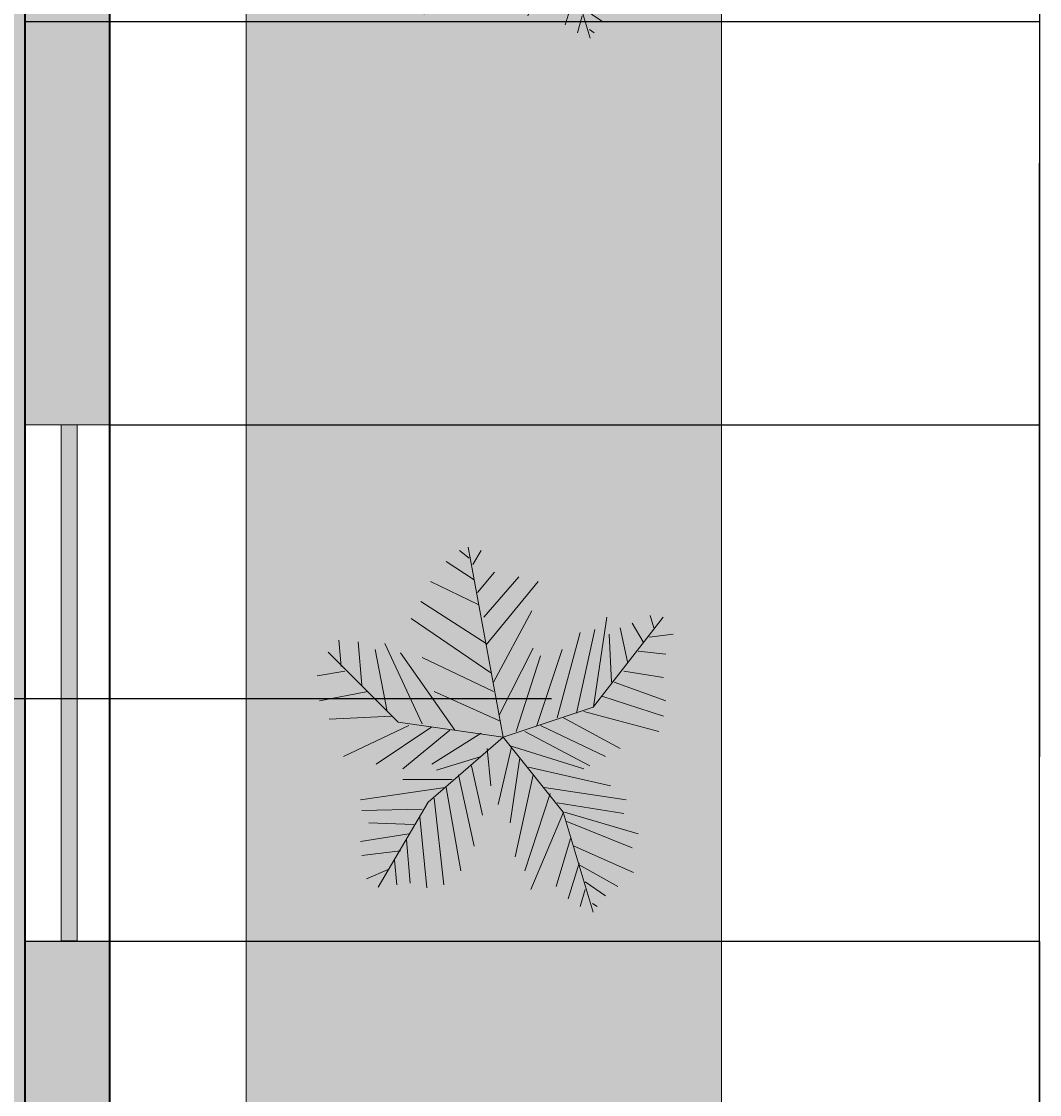
# Model space of a CAD drawing. Units: millimetres. Extents: x -229 to 16545, y -10488 to 4272.
# Tile 25 of 29: x 13776 to 16545, y -4126 to -1208. Entities that reach past the tile are written whole.
import ezdxf

# ---------------------------------------------------------------- set-up
doc = ezdxf.new("R2010")
doc.units = ezdxf.units.MM
for name, color, linetype, lineweight in [('A-ANNO-DIMS', 2, 'Continuous', 18), ('A-GLAZ', 4, 'Continuous', 18), ('A-WALL', 7, 'Continuous', 35), ('L-PLNT-BEDS', 82, 'Continuous', 18), ('L-PLNT-TREE', 80, 'Continuous', 18)]:
    doc.layers.add(name, color=color, linetype=linetype, lineweight=lineweight)
for name, color, linetype, lineweight, true_color in [('A-FLOR-PATT', 254, 'Continuous', 13, 0xfeeab9), ('A-WALL-PATT', 18, 'Continuous', 13, 0x000000), ('L-PLNT-PATT', 116, 'Continuous', 13, 0x136734)]:
    doc.layers.add(name, color=color, linetype=linetype, lineweight=lineweight, true_color=true_color)
doc.styles.get("Standard").update_dxf_attribs({"font": 'arial.ttf'})
doc.dimstyles.get("Standard").update_dxf_attribs({"dimtxt": 0.18, "dimasz": 0.18, "dimexe": 0.18, "dimexo": 0.0625, "dimgap": 0.09, "dimtad": 0, "dimtih": 1, "dimtoh": 1, "dimdec": 4, "dimzin": 0, "dimdsep": 46, "dimtxsty": 'Standard', "dimcen": 0.09, "dimadec": 0, "dimazin": 0, "dimtfac": 1, "dimtdec": 4, "dimtofl": 0, "dimtmove": 0, "dimatfit": 3, "dimfxl": 1, "dimtolj": 1, "dimtzin": 0, "dimarcsym": 0})

# ---------------------------------------------------------------- blocks, each defined once
blk = doc.blocks.new('*U18')
for p, q in [((-10.186, 53.64), (-13.084, 55.962)), ((0, 0), (-10.5, 57)), ((-9.099, 51.782), (-6.563, 55.962)), ((-8.737, 47.138), (-17.069, 52.711)), ((-7.65, 43.423), (-2.578, 49.46)), ((-7.288, 39.707), (-21.778, 46.673)), ((-5.839, 35.992), (4.667, 48.067)), ((-5.114, 27.632), (10.463, 46.673)), ((-5.114, 28.097), (-24.676, 40.636)), ((-3.665, 19.273), (-27.574, 35.527)), ((-2.941, 16.486), (8.652, 37.85)), ((27, 9), (48, 36)), ((27.127, 9.056), (31.112, 35.992)), ((44.153, 36.456), (45.239, 32.741)), ((22.055, 7.198), (27.489, 32.277)), ((35.096, 32.741), (37.27, 22.524)), ((38.719, 34.134), (41.979, 28.561)), ((-48.585, 21.131), (-49.309, 29.026)), ((16.259, 5.805), (23.142, 31.348)), ((31.836, 30.883), (32.561, 16.486)), ((43.791, 29.954), (51.036, 30.883)), ((-43.513, 28.561), (-42.427, 15.558)), ((-38.442, 26.239), (-34.819, 7.663)), ((-35.544, 28.097), (-24.314, 3.947)), ((-1.129, 6.734), (9.014, 26.704)), ((10.101, 3.483), (17.708, 26.239)), ((40.53, 25.775), (48.862, 24.846)), ((-31.5, 4.5), (-52.5, 25.5)), ((-14.533, 2.09), (-30.834, 25.31)), ((-24.314, 23.917), (-2.941, 13.7)), ((3.942, 1.625), (11.187, 24.381)), ((-47.498, 19.737), (-55.83, 18.344)), ((36.183, 19.737), (48.137, 17.88)), ((33.285, 16.486), (48.862, 10.913)), ((-40.615, 13.7), (-55.105, 10.913)), ((-20.691, 13.7), (-1.129, 4.876)), ((29.662, 12.307), (48.137, 6.269)), ((0, 0), (27, 9)), ((24.229, 7.663), (46.688, 1.625)), ((-33.37, 6.269), (-52.207, 5.34)), ((-28.299, 3.483), (-47.86, -5.805)), ((0, 0), (-31.5, 4.5)), ((11.187, 3.483), (30.749, -5.805)), ((18.07, 5.805), (35.096, -3.483)), ((-21.416, 3.018), (-38.079, -8.128)), ((-15.982, 2.09), (-30.11, -9.521)), ((0, 0), (-22.5, -19.5)), ((-6.563, 1.161), (-21.416, -8.128)), ((0, 0), (18, -22.5)), ((6.478, 1.625), (26.04, -8.592)), ((2.493, -3.019), (-1.491, -20.202)), ((1.769, -2.555), (24.229, -9.521)), ((-6.563, -5.805), (-19.967, -9.985)), ((-4.752, -3.483), (-3.665, -14.629)), ((5.029, -6.27), (2.131, -25.775)), ((-9.461, -8.592), (-6.201, -23.453)), ((7.565, -9.056), (32.198, -14.629)), ((-15.257, -12.772), (-30.11, -12.772)), ((-13.446, -11.378), (-8.737, -32.741)), ((9.014, -11.378), (3.58, -35.992)), ((-17.431, -15.094), (-42.789, -18.809)), ((-17.069, -15.094), (-12.721, -40.172)), ((12.274, -15.094), (36.907, -18.809)), ((-20.691, -18.345), (-17.793, -44.352)), ((14.085, -16.951), (6.478, -40.172)), ((-24.314, -21.596), (-42.427, -22.06)), ((-22.5, -19.5), (-37.5, -45)), ((18.07, -22.524), (8.289, -45.745)), ((16.259, -19.738), (36.183, -22.989)), ((18, -22.5), (27, -52.5)), ((18.433, -22.524), (40.53, -29.026)), ((-25.038, -23.918), (-22.865, -45.281)), ((19.157, -25.311), (38.719, -33.206)), ((-26.849, -26.24), (-40.253, -25.775)), ((-28.299, -29.026), (-42.789, -31.348)), ((-29.023, -30.884), (-27.936, -43.887)), ((20.244, -30.419), (15.897, -44.816)), ((-30.834, -34.135), (-42.427, -35.528)), ((21.331, -32.741), (39.081, -40.636)), ((-32.646, -36.921), (-31.921, -44.352)), ((22.78, -37.85), (19.519, -48.532)), ((22.78, -38.314), (34.372, -44.816)), ((-34.457, -39.708), (-40.978, -42.494)), ((24.591, -43.423), (30.749, -47.603)), ((24.591, -45.745), (23.142, -50.854)), ((26.764, -49.925), (28.213, -50.854))]:
    blk.add_line(p, q)
blk = doc.blocks.new('*D48')
at = {"layer": 'A-ANNO-DIMS', "color": 0, "lineweight": -2, "transparency": 16777216}
for p, q in [((14016, 2251.7), (16544.5, 2251.7)), ((16544.3, 2251.5), (16544.3, -1593.1)), ((16544.3, -5438.1), (16544.3, -1593.5)), ((13786, -5438.3), (16544.5, -5438.3))]:
    blk.add_line(p, q, dxfattribs=at)
at = {"layer": 'A-ANNO-DIMS', "color": 0, "transparency": 16777216}
for points in [[(16544.3, 2251.5), (16544.4, 2251.5), (16544.3, 2251.7)], [(16544.3, -5438.1), (16544.4, -5438.1), (16544.3, -5438.3)]]:
    blk.add_solid(points, dxfattribs=at)
at = {"layer": 'Defpoints', "color": 0, "transparency": 16777216}
for p in [(14015.9, 2251.7), (13785.9, -5438.3), (16544.3, -5438.3)]:
    blk.add_point(p, dxfattribs=at)
at = {"layer": 'A-ANNO-DIMS', "color": 0, "transparency": 16777216, "insert": (16544.3, -1593.3), "char_height": 0.18, "attachment_point": 5}
blk.add_mtext('\\A1;7690', dxfattribs=at)
blk = doc.blocks.new('*D57')
at = {"layer": 'A-ANNO-DIMS', "color": 0, "lineweight": -2, "transparency": 16777216}
for p, q in [((13786, -1208.3), (16544.5, -1208.3)), ((16544.3, -1208.5), (16544.3, -3208.1)), ((16544.3, -5208.1), (16544.3, -3208.5)), ((13786, -5208.3), (16544.5, -5208.3))]:
    blk.add_line(p, q, dxfattribs=at)
at = {"layer": 'A-ANNO-DIMS', "color": 0, "transparency": 16777216}
for points in [[(16544.3, -1208.5), (16544.4, -1208.5), (16544.3, -1208.3)], [(16544.3, -5208.1), (16544.4, -5208.1), (16544.3, -5208.3)]]:
    blk.add_solid(points, dxfattribs=at)
at = {"layer": 'Defpoints', "color": 0, "transparency": 16777216}
for p in [(13785.9, -1208.3), (13785.9, -5208.3), (16544.3, -5208.3)]:
    blk.add_point(p, dxfattribs=at)
at = {"layer": 'A-ANNO-DIMS', "color": 0, "transparency": 16777216, "insert": (16544.3, -3208.3), "char_height": 0.18, "attachment_point": 5}
blk.add_mtext('\\A1;4000', dxfattribs=at)
blk = doc.blocks.new('*D74')
at = {"layer": 'A-ANNO-DIMS', "color": 0, "lineweight": -2, "transparency": 16777216}
for p, q in [((14016, -2305.5), (16544.5, -2305.5)), ((16544.3, -2305.6), (16544.3, -3007.3)), ((16544.3, -3709.4), (16544.3, -3007.7)), ((14016, -3709.5), (16544.5, -3709.5))]:
    blk.add_line(p, q, dxfattribs=at)
at = {"layer": 'A-ANNO-DIMS', "color": 0, "transparency": 16777216}
for points in [[(16544.3, -2305.6), (16544.4, -2305.6), (16544.3, -2305.5)], [(16544.3, -3709.4), (16544.4, -3709.4), (16544.3, -3709.5)]]:
    blk.add_solid(points, dxfattribs=at)
at = {"layer": 'Defpoints', "color": 0, "transparency": 16777216}
for p in [(14015.9, -2305.5), (14015.9, -3709.5), (16544.3, -3709.5)]:
    blk.add_point(p, dxfattribs=at)
at = {"layer": 'A-ANNO-DIMS', "color": 0, "transparency": 16777216, "insert": (16544.3, -3007.5), "char_height": 0.18, "attachment_point": 5}
blk.add_mtext('\\A1;1404', dxfattribs=at)
blk = doc.blocks.new('*D87')
at = {"layer": 'A-ANNO-DIMS', "color": 0, "lineweight": -2, "transparency": 16777216}
for p, q in [((13786, -3709.5), (16544.5, -3709.5)), ((16544.3, -3709.7), (16544.3, -4458.7)), ((16544.3, -5208.1), (16544.3, -4459.1)), ((13786, -5208.3), (16544.5, -5208.3))]:
    blk.add_line(p, q, dxfattribs=at)
at = {"layer": 'A-ANNO-DIMS', "color": 0, "transparency": 16777216}
for points in [[(16544.3, -3709.7), (16544.4, -3709.7), (16544.3, -3709.5)], [(16544.3, -5208.1), (16544.4, -5208.1), (16544.3, -5208.3)]]:
    blk.add_solid(points, dxfattribs=at)
at = {"layer": 'Defpoints', "color": 0, "transparency": 16777216}
for p in [(13785.9, -3709.5), (16544.3, -3709.5), (13785.9, -5208.3)]:
    blk.add_point(p, dxfattribs=at)
at = {"layer": 'A-ANNO-DIMS', "color": 0, "transparency": 16777216, "insert": (16544.3, -4458.9), "char_height": 0.18, "attachment_point": 5}
blk.add_mtext('\\A1;1498.7', dxfattribs=at)
blk = doc.blocks.new('*D101')
at = {"layer": 'A-ANNO-DIMS', "color": 0, "lineweight": -2, "transparency": 16777216}
for p, q in [((10907.8, -3049.7), (10908, -3049.7)), ((10907.9, -3049.8), (10907.9, -3049.6)), ((15176.9, -3049.7), (13576.2, -3049.7))]:
    blk.add_line(p, q, dxfattribs=at)
at = {"layer": 'A-ANNO-DIMS', "color": 0, "transparency": 16777216}
blk.add_solid([(13576.2, -3049.7), (13576.2, -3049.7), (13576, -3049.7)], dxfattribs=at)
at = {"layer": 'Defpoints', "color": 0, "transparency": 16777216}
for p in [(10907.9, -3049.7), (13576, -3049.7)]:
    blk.add_point(p, dxfattribs=at)
at = {"layer": 'A-ANNO-DIMS', "color": 0, "transparency": 16777216, "insert": (15177.3, -3049.7), "char_height": 0.18, "attachment_point": 5}
blk.add_mtext('\\A1;R2668', dxfattribs=at)
blk = doc.blocks.new('*D102')
at = {"layer": 'A-ANNO-DIMS', "color": 0, "lineweight": -2, "transparency": 16777216}
for p, q in [((11192.8, -3049.7), (11193, -3049.7)), ((11192.9, -3049.8), (11192.9, -3049.6)), ((15217.2, -3049.7), (13708.3, -3049.7))]:
    blk.add_line(p, q, dxfattribs=at)
at = {"layer": 'A-ANNO-DIMS', "color": 0, "transparency": 16777216}
blk.add_solid([(13708.3, -3049.7), (13708.3, -3049.7), (13708.1, -3049.7)], dxfattribs=at)
at = {"layer": 'Defpoints', "color": 0, "transparency": 16777216}
for p in [(11192.9, -3049.7), (13708.1, -3049.7)]:
    blk.add_point(p, dxfattribs=at)
at = {"layer": 'A-ANNO-DIMS', "color": 0, "transparency": 16777216, "insert": (15217.6, -3049.7), "char_height": 0.18, "attachment_point": 5}
blk.add_mtext('\\A1;R2515', dxfattribs=at)

msp = doc.modelspace()

# ---------------------------------------------------------------- hatches: boundary and pattern name
at = {"layer": 'A-FLOR-PATT', "transparency": 33554592}
h = msp.add_hatch(color=256, dxfattribs=at)
h.dxf.hatch_style = 1
h.paths.add_polyline_path([(7975.933, -5325.772), (7943.121, -5325.772), (7943.121, -4576.49, 0.40145271), (7225.933, -5325.772, 0.40145271), (6508.746, -4576.49), (6508.746, -5325.772), (6475.933, -5325.772), (6475.933, -5438.272), (5975.933, -5438.272), (5975.933, -7267.724), (5975.933, -7438.272), (6478.619, -7438.272), (6463.448, -7355.919), (6464.88, -7356.837), (6463.849, -7358.097), (6478.619, -7438.272), (6610.327, -7438.272), (6632.656, -7409.564), (6632.525, -7406.967), (6634.208, -7407.569), (6619.273, -7426.77), (6654.466, -7438.272), (7610.517, -7438.272), (7607.41, -7421.409), (7608.842, -7422.327), (7607.812, -7423.587), (7610.517, -7438.272), (7975.933, -7438.272)])
h.paths.add_polyline_path([(13785.933, -1208.272), (9555.933, -1208.272), (9555.933, -961.785), (9705.933, -961.785), (9705.933, -918.035), (10704.976, -918.035, 0.40145271), (9705.933, 38.215), (9555.933, 38.215), (9555.933, 2021.728), (5975.933, 2021.728), (5975.933, 755.492), (5745.933, 755.492), (5745.933, 1427.266), (2918.813, 1427.266), (2918.813, -492.942), (5013.319, -492.942), (5013.319, -978.272), (5745.933, -978.272), (5745.933, -397.513), (5975.933, -397.513), (5975.933, -1208.272), (4560.933, -1208.272), (4560.933, -1265.772), (4448.433, -1265.772), (4448.433, -1298.585), (4445.933, -1298.585), (3699.151, -1298.585, 0.40145271), (4448.433, -2015.772), (4560.933, -2015.772), (4560.933, -2384.177), (5745.933, -2384.177), (5799.402, -2384.177), (5799.402, -4518.272), (5975.933, -4518.272), (5975.933, -5208.272), (6475.933, -5208.272), (6475.933, -4575.772), (6508.746, -4575.772), (6508.746, -4576.49, -0.35647263), (7216.672, -5208.272), (7235.194, -5208.272, -0.35647263), (7943.121, -4576.49), (7943.121, -4575.772), (7975.933, -4575.772), (7975.933, -5208.272), (11176.247, -5208.272), (11159.44, -5191.465), (10520.768, -5191.465), (10520.768, -4888.936), (10571.19, -4888.936), (10571.19, -4872.129), (10772.876, -4872.129), (10772.876, -4888.936), (10789.683, -4888.936), (10789.683, -4872.129), (10991.368, -4872.129), (10991.368, -4888.936), (11041.79, -4888.936), (11041.79, -4872.129), (11058.597, -4872.129, -0.09090909), (11428.354, -4872.129), (11445.162, -4872.129), (11445.162, -4888.936), (11529.197, -4888.936), (11529.197, -5191.465), (11327.512, -5191.465), (11310.704, -5208.272), (13785.933, -5208.272)])
h.paths.add_polyline_path([(11047.216, -1630.944, -1), (11402.816, -1630.944, -1)], flags=16)
h.paths.add_polyline_path([(11148.816, -1630.944), (11225.016, -1554.744), (11301.216, -1630.944), (11225.016, -1707.144)], flags=0)
h.paths.add_polyline_path([(11199.616, -1630.944, -1), (11250.416, -1630.944, -1)], flags=0)
h.paths.add_polyline_path([(11588.751, -2096.259), (11588.751, -1543.254, -0.26666697), (12864.918, -1543.254), (12864.918, -2096.259), (12737.302, -2096.259), (12737.302, -2063.121), (11716.368, -2063.121), (11716.368, -2096.259)], flags=16)
h.paths.add_polyline_path([(12012.696, -2489.42), (12600.997, -2489.42), (12600.997, -3666.022), (12012.696, -3666.022)], flags=16)
h.paths.add_polyline_path([(12176.41, -3599.403), (12174.938, -3609.076), (12173.789, -3618.819), (12173.09, -3628.559), (12172.973, -3638.221), (12173.89, -3652.852), (12175.008, -3657.025), (12172.909, -3643.473), (12173.142, -3624.297), (12175.386, -3605.273)], flags=0)
h.paths.add_polyline_path([(8026.289, -286.944), (7737.703, -287.19), (7734.87, -269.156), (8029.092, -268.905)], flags=16)
h.paths.add_polyline_path([(7733.453, -260.139), (7710.784, -115.865), (7557.191, -115.996), (7556.999, 109.744), (7412.687, 132.166), (7412.433, 429.206), (7556.707, 451.876), (7556.568, 614.769), (7412.256, 637.19), (7412.003, 934.231), (7556.276, 956.9), (7556.084, 1182.639), (7709.677, 1182.77), (7732.099, 1327.082), (8029.14, 1327.335), (8051.808, 1183.062), (8205.401, 1183.192), (8205.594, 957.454), (8349.906, 935.031), (8350.159, 637.99), (8205.885, 615.322), (8206.024, 452.43), (8350.336, 430.006), (8350.59, 132.965), (8206.316, 110.298), (8206.509, -115.442), (8052.916, -115.573), (8030.493, -259.885)], flags=16)
h.paths.add_polyline_path([(12261.416, -3475.554), (12262.632, -3486.776), (12264.032, -3497.007), (12265.554, -3506.365), (12267.136, -3514.968), (12268.719, -3522.935), (12271.304, -3535.59), (12273.606, -3548.078), (12275.271, -3561.064), (12275.93, -3574.938), (12275.325, -3590.3), (12273.425, -3607.964), (12270.795, -3625.658), (12268.066, -3641.063), (12266.318, -3649.679), (12265.456, -3653.626), (12263.984, -3659.846), (12264.032, -3659.566), (12264.342, -3658.241), (12264.807, -3656.37), (12265.456, -3653.626), (12266.318, -3649.679), (12267.409, -3644.302), (12268.668, -3637.664), (12270.019, -3630.037), (12271.384, -3621.695), (12272.69, -3612.908), (12273.857, -3603.948), (12274.81, -3595.088), (12275.47, -3586.601), (12275.782, -3578.689), (12275.757, -3571.292), (12275.423, -3564.275), (12274.816, -3557.512), (12273.964, -3550.872), (12272.896, -3544.224), (12271.645, -3537.439), (12270.24, -3530.385), (12267.543, -3517.181), (12264.612, -3501.247), (12261.849, -3481.059)], flags=0)
h.paths.add_polyline_path([(12332.136, -3408.03), (12333.483, -3416.79), (12335.077, -3424.54), (12336.915, -3431.355), (12338.991, -3437.32), (12341.266, -3442.55), (12343.694, -3447.166), (12346.229, -3451.292), (12348.826, -3455.051), (12351.438, -3458.563), (12357.476, -3466.491), (12363.61, -3476.575), (12368.309, -3489.762), (12369.929, -3503.427), (12369.842, -3516.511), (12368.43, -3530.867), (12365.816, -3545.835), (12362.382, -3559.786), (12360.968, -3564.487), (12363.063, -3557.021), (12364.898, -3549.566), (12366.473, -3542.077), (12367.773, -3534.631), (12368.781, -3527.301), (12369.483, -3520.162), (12369.863, -3513.291), (12369.906, -3506.759), (12369.599, -3500.643), (12368.93, -3494.999), (12367.924, -3489.796), (12366.61, -3484.994), (12365.024, -3480.542), (12363.19, -3476.399), (12361.141, -3472.516), (12358.909, -3468.847), (12356.525, -3465.347), (12354.02, -3461.954), (12351.438, -3458.563), (12345.462, -3450.529), (12339.923, -3439.996), (12335.85, -3428.296), (12332.68, -3412.888)], flags=0)
h.paths.add_polyline_path([(12385.287, -3334.612), (12384.977, -3342.409), (12385.02, -3349.196), (12385.4, -3355.066), (12386.104, -3360.105), (12387.112, -3364.41), (12388.412, -3368.071), (12389.987, -3371.181), (12391.823, -3373.832), (12393.919, -3376.097), (12396.337, -3377.978), (12399.153, -3379.462), (12402.445, -3380.531), (12406.289, -3381.172), (12410.758, -3381.371), (12415.935, -3381.106), (12421.893, -3380.368), (12428.658, -3379.159), (12436.069, -3377.55), (12443.907, -3375.635), (12451.961, -3373.505), (12460.015, -3371.254), (12467.853, -3368.971), (12475.263, -3366.749), (12482.029, -3364.68), (12491.877, -3361.657), (12497.701, -3360.107), (12501.639, -3359.288), (12510.135, -3358.326), (12519.662, -3365.412), (12524.243, -3378.911), (12523.764, -3390.7), (12520.746, -3401.577), (12514.248, -3415.634), (12511.518, -3420.418), (12515.856, -3412.154), (12519.153, -3405.024), (12521.516, -3398.804), (12523.049, -3393.276), (12523.865, -3388.212), (12524.059, -3383.441), (12523.7, -3378.958), (12522.853, -3374.815), (12521.576, -3371.054), (12519.931, -3367.722), (12517.982, -3364.865), (12515.786, -3362.529), (12513.405, -3360.758), (12510.877, -3359.588), (12508.136, -3358.982), (12505.086, -3358.897), (12501.639, -3359.288), (12497.701, -3360.107), (12493.183, -3361.309), (12487.988, -3362.851), (12476.403, -3366.408), (12463.335, -3370.326), (12447.372, -3374.788), (12431.759, -3378.604), (12418.504, -3380.974), (12405.811, -3381.624), (12394.725, -3378.025), (12388.039, -3368.367), (12385.583, -3357.877), (12384.826, -3346.204), (12385.428, -3331.059), (12385.953, -3325.719)], flags=0)
h.paths.add_polyline_path([(7880.016, 1173.969), (7880.373, 1175.495), (7880.433, 1175.851), (7879.484, 1171.818)], flags=0)
h.paths.add_polyline_path([(7802.33, 874.962), (7800.771, 885.032), (7798.932, 893.941), (7796.811, 901.774), (7794.419, 908.63), (7791.798, 914.639), (7789.002, 919.945), (7786.083, 924.686), (7783.093, 929.005), (7780.087, 933.043), (7774.996, 939.717), (7768.406, 949.37), (7762.174, 963.427), (7759.342, 978.002), (7758.629, 991.888), (7759.492, 1007.928), (7761.801, 1025.496), (7765.392, 1044.035), (7766.625, 1049.048), (7764.522, 1039.543), (7762.719, 1030.232), (7761.232, 1021.168), (7760.08, 1012.405), (7759.28, 1003.994), (7758.849, 995.988), (7758.806, 988.44), (7759.167, 981.404), (7759.942, 974.914), (7761.104, 968.936), (7762.617, 963.414), (7764.448, 958.299), (7766.559, 953.535), (7768.918, 949.073), (7771.487, 944.856), (7774.232, 940.835), (7777.115, 936.938), (7782.377, 930.041), (7787.845, 922.139), (7793.348, 911.698), (7798.042, 898.247), (7801.702, 880.527)], flags=0)
h.paths.add_polyline_path([(12519.068, -3228.534), (12519.615, -3236.235), (12520.529, -3242.343), (12521.78, -3247.103), (12523.337, -3250.758), (12525.171, -3253.556), (12527.248, -3255.709), (12529.522, -3257.296), (12531.95, -3258.361), (12534.486, -3258.949), (12537.082, -3259.11), (12539.694, -3258.888), (12542.277, -3258.329), (12544.781, -3257.478), (12547.173, -3256.388), (12549.46, -3255.129), (12550.455, -3254.517), (12555.825, -3251.109), (12557.835, -3249.942), (12565.181, -3246.404), (12574.565, -3253.032), (12576.931, -3265.022), (12576.627, -3277.425), (12575.416, -3290.819), (12574.851, -3295.392), (12575.708, -3287.593), (12576.322, -3280.806), (12576.688, -3274.939), (12576.812, -3269.899), (12576.688, -3265.593), (12576.322, -3261.932), (12575.708, -3258.822), (12574.851, -3256.172), (12573.753, -3253.905), (12572.439, -3252.005), (12570.943, -3250.474), (12569.293, -3249.309), (12567.523, -3248.513), (12565.658, -3248.083), (12563.732, -3248.022), (12561.777, -3248.328), (12559.814, -3248.989), (12557.835, -3249.942), (12555.825, -3251.109), (12553.77, -3252.413), (12551.652, -3253.78), (12549.46, -3255.129), (12543.167, -3258.594), (12532.661, -3259.485), (12524.685, -3253.923), (12520.949, -3245.152), (12519.138, -3233.042)], flags=0)
h.paths.add_polyline_path([(7741.293, 790.501), (7741.641, 799.467), (7741.584, 807.269), (7741.141, 814.015), (7740.329, 819.809), (7739.165, 824.757), (7737.667, 828.966), (7735.853, 832.541), (7733.74, 835.586), (7731.348, 838.188), (7728.71, 840.348), (7725.861, 842.052), (7722.836, 843.28), (7719.671, 844.015), (7716.4, 844.237), (7713.06, 843.932), (7709.684, 843.081), (7706.304, 841.686), (7702.923, 839.834), (7699.543, 837.629), (7696.164, 835.178), (7692.784, 832.585), (7684.718, 826.315), (7675.609, 820.63), (7664.001, 817.274), (7654.105, 821.884), (7647.171, 832.02), (7644.191, 846.522), (7646.321, 860.288), (7647.49, 864.223), (7645.946, 857.865), (7645.046, 852.044), (7644.827, 846.557), (7645.243, 841.404), (7646.221, 836.642), (7647.693, 832.318), (7649.587, 828.489), (7651.832, 825.206), (7654.359, 822.523), (7657.097, 820.49), (7659.984, 819.145), (7662.993, 818.452), (7666.108, 818.357), (7669.311, 818.809), (7672.583, 819.755), (7675.908, 821.139), (7679.268, 822.913), (7682.645, 825.021), (7686.025, 827.401), (7689.404, 829.958), (7692.784, 832.585), (7700.505, 838.509), (7709.871, 843.64), (7721.436, 844.698), (7733.277, 837.617), (7739.571, 825.214), (7741.557, 811.049), (7741.669, 795.575)], flags=0)
h.paths.add_polyline_path([(8377.641, 137.216), (8359.607, 134.382), (8359.356, 428.605), (8377.395, 425.802)], flags=16)
h.paths.add_polyline_path([(7650.715, 668.465), (7650.08, 677.319), (7649.023, 684.34), (7647.579, 689.811), (7645.785, 694.012), (7643.675, 697.228), (7641.286, 699.7), (7638.669, 701.521), (7635.876, 702.744), (7632.96, 703.419), (7629.974, 703.601), (7626.971, 703.344), (7624.004, 702.697), (7621.125, 701.717), (7618.375, 700.462), (7615.749, 699.013), (7614.561, 698.279), (7608.435, 694.382), (7606.125, 693.04), (7598.981, 689.594), (7589.669, 693.773), (7585.26, 702.856), (7584.221, 713.11), (7584.49, 724.584), (7585.863, 739.937), (7586.518, 745.277), (7585.539, 736.31), (7584.841, 728.507), (7584.424, 721.761), (7584.288, 715.966), (7584.433, 711.016), (7584.86, 706.807), (7585.567, 703.231), (7586.556, 700.186), (7587.821, 697.58), (7589.332, 695.397), (7591.053, 693.637), (7592.951, 692.3), (7594.989, 691.385), (7597.132, 690.895), (7599.346, 690.826), (7601.594, 691.18), (7603.851, 691.943), (7606.125, 693.04), (7608.435, 694.382), (7610.797, 695.885), (7613.229, 697.458), (7620.475, 701.929), (7632.001, 704.44), (7643.476, 699.417), (7648.536, 687.571), (7650.63, 673.661)], flags=0)
h.paths.add_polyline_path([(7385.628, 136.37), (7385.382, 424.956), (7403.416, 427.789), (7403.667, 133.567)], flags=16)
h.paths.add_polyline_path([(12993.884, -2257.186), (12959.588, -2257.186), (12959.588, -2125.099), (13531.966, -2125.099, -0.19047621), (13531.966, -3974.321), (12959.588, -3974.321), (12959.588, -3842.233), (12993.884, -3842.233)], flags=16)
h.paths.add_polyline_path([(13413.486, -3313.884), (13413.486, -2785.535), (13562.885, -2785.535, -0.04962821), (13562.885, -3313.884)], flags=0)
h.paths.add_polyline_path([(8377.21, 642.241), (8359.176, 639.407), (8358.925, 933.629), (8376.964, 930.826)], flags=16)
h.paths.add_polyline_path([(13086.058, -1864.83), (13086.058, -1449.84), (13501.048, -1449.84), (13501.048, -1864.83)], flags=16)
h.paths.add_polyline_path([(13305.814, -1862.197), (13302.103, -1859.624), (13298.088, -1857.068), (13293.799, -1854.536), (13289.262, -1852.031), (13284.504, -1849.559), (13279.554, -1847.125), (13274.439, -1844.735), (13269.17, -1842.389), (13263.701, -1840.081), (13257.97, -1837.797), (13251.914, -1835.525), (13245.472, -1833.252), (13238.582, -1830.968), (13231.18, -1828.66), (13223.206, -1826.315), (13209.182, -1822.458), (13204.584, -1821.48), (13217.962, -1824.773), (13235.072, -1829.804), (13248.777, -1834.349), (13260.829, -1838.869), (13274.479, -1844.63), (13289.675, -1852.101), (13302.553, -1859.704)], flags=0)
h.paths.add_polyline_path([(13428.104, -1820.994), (13419.007, -1818.141), (13409.95, -1815.4), (13400.766, -1812.747), (13391.271, -1810.151), (13376.087, -1806.251), (13370.618, -1805.019), (13386.304, -1808.794), (13405.087, -1813.928), (13423.014, -1819.354)], flags=0)
h.paths.add_polyline_path([(7385.197, 641.395), (7384.951, 929.98), (7402.986, 932.814), (7403.236, 638.592)], flags=16)
h.paths.add_polyline_path([(13262.537, -1725.526), (13253.246, -1724.74), (13244.516, -1724.117), (13235.94, -1723.625), (13223.267, -1723.062), (13217.598, -1722.912), (13231.966, -1723.397), (13248.733, -1724.359), (13266.899, -1725.895), (13272.802, -1726.502)], flags=0)
h.paths.add_polyline_path([(13191.893, -1641.137), (13208.675, -1640.506), (13214.057, -1640.258), (13197.763, -1640.936)], flags=0)
h.paths.add_polyline_path([(13097.524, -1608.457), (13114.284, -1609.031), (13120.126, -1609.105), (13103.045, -1608.71)], flags=0)
h.paths.add_polyline_path([(13465.328, -1521.577), (13473.906, -1517.015), (13481.761, -1511.636), (13492.562, -1502.076), (13495.327, -1497.933), (13485.818, -1508.858), (13470.208, -1519.547)], flags=0)
h.paths.add_polyline_path([(13175.015, -1500.891), (13184.046, -1501.807), (13192.721, -1502.52), (13201.114, -1503.034), (13209.273, -1503.351), (13217.244, -1503.476), (13225.078, -1503.41), (13232.821, -1503.16), (13240.524, -1502.728), (13248.233, -1502.117), (13255.993, -1501.322), (13263.825, -1500.293), (13271.746, -1498.974), (13279.775, -1497.305), (13287.928, -1495.229), (13296.222, -1492.688), (13304.675, -1489.622), (13313.304, -1485.975), (13322.089, -1481.727), (13330.859, -1477.028), (13339.408, -1472.063), (13347.526, -1467.02), (13355.006, -1462.087), (13364.86, -1455.202), (13367.224, -1453.299), (13358.544, -1459.754), (13343.348, -1469.775), (13326.143, -1479.767), (13309.023, -1488.045), (13292.249, -1494.129), (13276.009, -1498.264), (13260.299, -1500.88), (13244.401, -1502.51), (13228.945, -1503.378), (13213.316, -1503.508), (13197.047, -1502.876), (13180.088, -1501.481)], flags=0)
h.paths.add_polyline_path([(7733.501, 1336.101), (7736.303, 1354.14), (8024.889, 1354.386), (8027.723, 1336.352)], flags=16)
at = {"layer": 'A-WALL-PATT'}
h = msp.add_hatch(color=256, dxfattribs=at)
h.dxf.hatch_style = 1
h.paths.add_polyline_path([(7294.425, 2163.983), (7294.425, 2251.728), (4412.722, 2251.728), (4412.722, 2166.741), (4412.722, 2122.457), (4412.722, 2021.728), (7294.425, 2021.728), (7294.425, 2119.698)])
h.paths.add_polyline_path([(11407.51, 2166.741), (11407.51, 2251.728), (8296.763, 2251.728), (8296.763, 2163.983), (8296.763, 2119.698), (8296.763, 2021.728), (11407.51, 2021.728), (11407.51, 2122.457)])
h.paths.add_polyline_path([(9785.933, 2021.728), (9555.933, 2021.728), (9555.933, 38.215), (9705.933, 38.215, -0.02002407), (9785.933, 35.01)])
h.paths.add_polyline_path([(14015.933, 2251.728), (12488.002, 2251.728), (12488.002, 2166.742), (12488.002, 2122.738), (12488.002, 2021.728), (13785.933, 2021.728), (13785.933, -2305.465), (13883.903, -2305.465), (13928.188, -2305.465), (14015.933, -2305.465)])
h.paths.add_polyline_path([(13785.933, -978.272), (9785.933, -978.272), (9785.933, -961.785), (9705.933, -961.785), (9555.933, -961.785), (9555.933, -1208.272), (13785.933, -1208.272)])
h.paths.add_polyline_path([(5975.933, 2021.728), (5745.933, 2021.728), (5745.933, 755.492), (5975.933, 755.492)])
h.paths.add_polyline_path([(2245.933, 2021.728), (3420.865, 2021.728), (3420.865, 2122.457), (3420.865, 2167.104), (3420.865, 2251.728), (2015.933, 2251.728), (2015.933, -3326.811), (2100.943, -3326.811), (2155.199, -3326.811), (2245.933, -3326.811)])
h.paths.add_polyline_path([(5975.933, -397.513), (5745.933, -397.513), (5745.933, -978.272), (2245.933, -978.272), (2245.933, -1208.272), (5975.933, -1208.272)])
h.paths.add_polyline_path([(12015.17, -5208.272), (7975.933, -5208.272), (7975.933, -5325.772), (7975.933, -5438.272), (7975.933, -5596.884), (8205.933, -5596.884), (8205.933, -5438.272), (12015.17, -5438.272), (12015.17, -5337.543), (12015.17, -5293.259)])
h.paths.add_polyline_path([(5975.933, -4518.272), (4567.83, -4518.272), (4567.83, -4603.259), (4567.83, -4647.543), (4567.83, -4748.272), (5745.933, -4748.272), (5745.933, -5438.272), (5975.933, -5438.272), (6475.933, -5438.272), (6475.933, -5325.772), (6475.933, -5208.272), (5975.933, -5208.272)])
h.paths.add_polyline_path([(3765.491, -4518.272), (2245.933, -4518.272), (2245.933, -4748.272), (3765.491, -4748.272), (3765.491, -4647.543), (3765.491, -4603.259)])
h = msp.add_hatch(color=256, dxfattribs=at)
h.dxf.hatch_style = 1
h.paths.add_polyline_path([(13883.903, -2305.465), (13928.188, -2305.465), (13928.188, -3709.532), (14015.933, -3709.532), (14015.933, -5692.852), (13785.933, -5692.852), (13785.933, -5438.272), (12817.508, -5438.272), (12817.508, -5337.543), (12015.17, -5337.543), (12015.17, -5293.259), (12817.508, -5293.259), (12817.508, -5208.272), (13785.933, -5208.272), (13785.933, -3709.532), (13883.903, -3709.532)])
at = {"layer": 'L-PLNT-PATT'}
h = msp.add_hatch(dxfattribs=at)
h.set_pattern_fill('GRASS', color=256, scale=2)
h.set_pattern_definition([(90, (-8141.222, -13125.504), (-35.921024, 35.921024), [9.525, -62.31705]), (45, (-8141.22, -13125.504), (-35.92102, 35.92102), [9.525, -41.275]), (135, (-8141.22, -13125.504), (-35.92102, -35.92102), [9.525, -41.275])])
h.paths.add_polyline_path([(15679.607, 2251.728), (14387.79, 2251.728), (14387.79, -7668.272), (8209.16, -7668.272), (8209.16, -9248.272), (14015.933, -9248.272), (15679.607, -9248.272)])

# ---------------------------------------------------------------- linework, layer by layer
at = {"layer": 'A-GLAZ'}
for p, q in [((13883.903, -2305.465), (13785.933, -2305.465)), ((13928.188, -2305.465), (14015.933, -2305.465)), ((13883.903, -3709.532), (13785.933, -3709.532)), ((13928.188, -3709.532), (14015.933, -3709.532))]:
    msp.add_line(p, q, dxfattribs=at)
msp.add_lwpolyline([(13928.188, -2305.465), (13928.188, -3708.357), (13883.903, -3708.357), (13883.903, -2305.465)], close=True, dxfattribs=at)
at = {"layer": 'A-WALL'}
for p, q in [((14015.933, 2251.728), (14015.933, -7438.272)), ((13785.933, 2021.728), (13785.933, -5208.272))]:
    msp.add_line(p, q, dxfattribs=at)
at = {"layer": 'L-PLNT-BEDS', "transparency": 33554572}
msp.add_line((14387.79, 2251.728), (14387.79, -7668.272), dxfattribs=at)
at = {"layer": 'L-PLNT-BEDS', "transparency": 33554554}
msp.add_line((15679.607, -9248.272), (15679.607, 2251.728), dxfattribs=at)

# ---------------------------------------------------------------- block references
at = {"layer": 'L-PLNT-TREE', "xscale": 9.061891725250485, "yscale": 9.061891725250485, "zscale": 9.061891725250485}
for p in [(15078.323, -778.078), (15086.156, -3154.043)]:
    msp.add_blockref('*U18', p, dxfattribs=at)

# ---------------------------------------------------------------- dimensions: what is measured, and where the dimension line sits
at = {"layer": 'A-ANNO-DIMS'}
for base, p1, p2, override, picture, middle in [((16544.342, -5438.272), (14015.933, 2251.728), (13785.933, -5438.272), {"dimdec": 0, "dimlfac": 1, "dimrnd": 0, "dimzin": 0, "dimdsep": 46, "dimlunit": 2}, '*D48', (16544.342, -1593.272)), ((16544.342, -5208.272), (13785.933, -1208.272), (13785.933, -5208.272), {"dimdec": 0, "dimlfac": 1, "dimrnd": 0, "dimzin": 0, "dimdsep": 46, "dimlunit": 2}, '*D57', (16544.342, -3208.272)), ((16544.342, -3709.532), (14015.933, -2305.465), (14015.933, -3709.532), {"dimdec": 0, "dimlfac": 1, "dimrnd": 0, "dimzin": 0, "dimdsep": 46, "dimlunit": 2}, '*D74', (16544.342, -3007.498)), ((16544.342, -3709.532), (13785.933, -5208.272), (13785.933, -3709.532), {"dimdec": 1, "dimlfac": 1, "dimrnd": 0, "dimzin": 0, "dimdsep": 46, "dimlunit": 2}, '*D87', (16544.342, -4458.902))]:
    dim = msp.add_linear_dim(base=base, p1=p1, p2=p2, angle=90, dimstyle='Standard', override=override, dxfattribs=at)
    dim.commit()
    dim.dimension.update_dxf_attribs({"geometry": picture, "text_midpoint": middle})
for center, mpoint, picture, middle in [((10907.903, -3049.71), (13575.995, -3049.709), '*D101', (15176.85, -3049.708)), ((11192.921, -3049.71), (13708.082, -3049.71), '*D102', (15217.179, -3049.71))]:
    dim = msp.add_radius_dim(center=center, mpoint=mpoint, dimstyle='Standard', override={"dimdec": 0, "dimlfac": 1, "dimrnd": 0, "dimzin": 0, "dimdsep": 46, "dimlunit": 2}, dxfattribs=at)
    dim.commit()
    dim.dimension.update_dxf_attribs({"geometry": picture, "text_midpoint": middle, "dimtype": 164})

doc.saveas('drawing.dxf')
